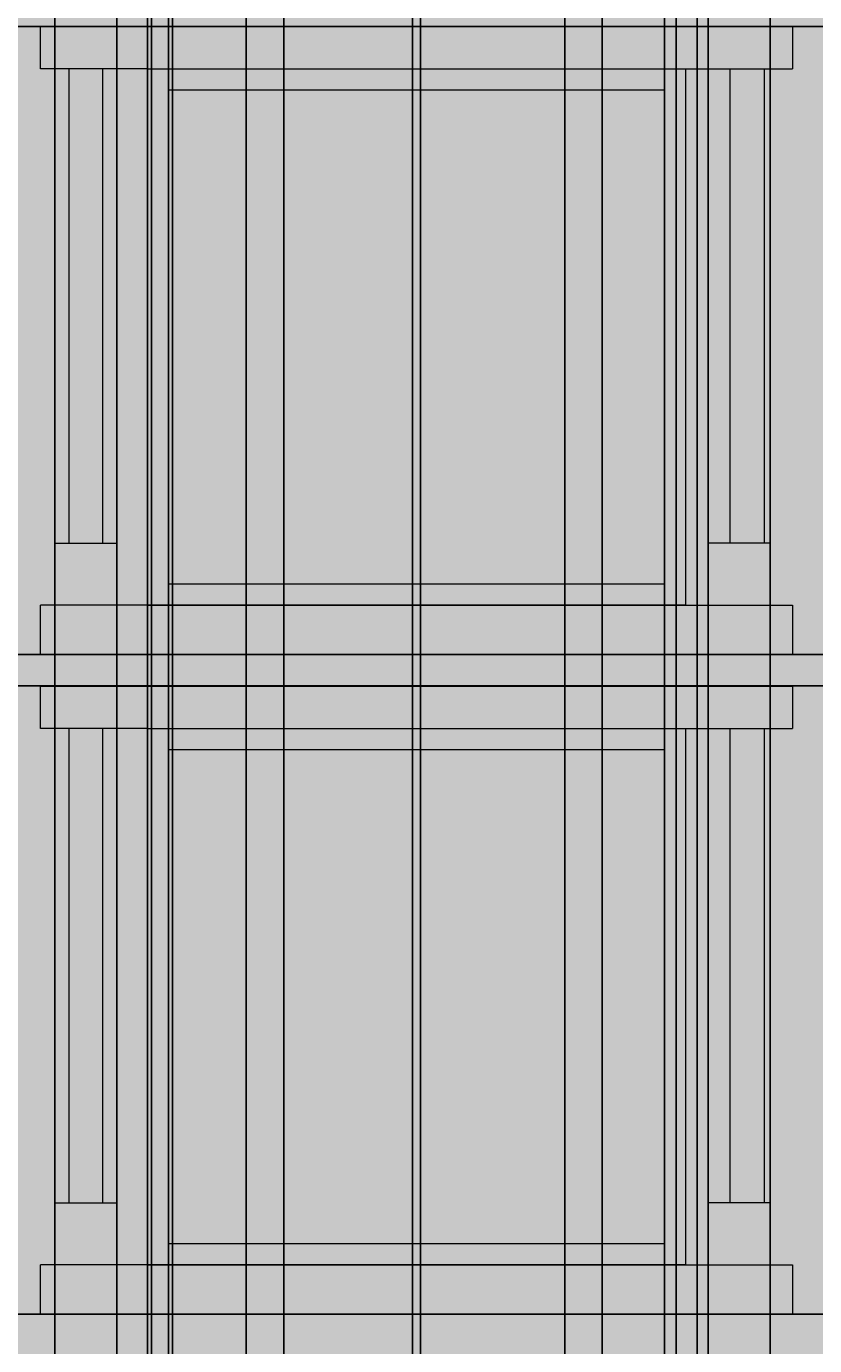
# Model space of a CAD drawing. Units: inches. Extents: x 3024 to 4744, y 1110 to 2100.
# Tile 12 of 29: x 3146 to 3297, y 1402 to 1654. Entities that reach past the tile are written whole.
import ezdxf

# ---------------------------------------------------------------- set-up
doc = ezdxf.new("R2010")
doc.units = ezdxf.units.IN
for name, color, linetype, lineweight in [('A-ANNO-DIMS', 2, 'Continuous', 18), ('A-ELEV', 7, 'Continuous', 25), ('A-ELEV-PATT', 252, 'Continuous', 13), ('A-GLAZ', 4, 'Continuous', 18)]:
    doc.layers.add(name, color=color, linetype=linetype, lineweight=lineweight)
doc.styles.get("Standard").update_dxf_attribs({"font": 'arial.ttf'})
doc.dimstyles.get("Standard").update_dxf_attribs({"dimtxt": 0.18, "dimasz": 0.18, "dimexe": 0.18, "dimexo": 0.0625, "dimgap": 0.09, "dimtad": 0, "dimtih": 1, "dimtoh": 1, "dimdec": 1, "dimzin": 0, "dimdsep": 46, "dimlunit": 3, "dimtxsty": 'Standard', "dimcen": 0.09, "dimadec": 0, "dimazin": 0, "dimtfac": 1, "dimtdec": 1, "dimtofl": 0, "dimtmove": 0, "dimatfit": 3, "dimfxl": 1, "dimtolj": 1, "dimtzin": 0, "dimarcsym": 0})

# ---------------------------------------------------------------- blocks, each defined once
blk = doc.blocks.new('WIN-BALCONY-A')
for p, q in [((3169.4, 1897.49), (3148.97, 1897.49)), ((3169.4, 1897.49), (3148.97, 1897.49)), ((3169.4, 1897.49), (3292.61, 1897.49)), ((3169.4, 1897.49), (3292.61, 1897.49)), ((3169.4, 1795.04), (3148.97, 1795.04)), ((3169.4, 1795.04), (3148.97, 1795.04)), ((3169.4, 1795.04), (3292.61, 1795.04)), ((3169.4, 1795.04), (3292.61, 1795.04))]:
    blk.add_line(p, q)
for points in [[(3148.97, 1897.49), (3148.97, 1905.61), (3292.61, 1905.61), (3292.61, 1897.49)], [(3148.97, 1897.49), (3148.97, 1905.61), (3292.61, 1905.61), (3292.61, 1897.49)], [(3292.61, 1795.04), (3292.61, 1785.61), (3148.97, 1785.61), (3148.97, 1795.04)], [(3292.61, 1795.04), (3292.61, 1785.61), (3148.97, 1785.61), (3148.97, 1795.04)]]:
    blk.add_lwpolyline(points)
for points in [[(3154.33, 1806.87), (3160.86, 1806.87), (3160.86, 1897.49), (3154.33, 1897.49)], [(3154.33, 1806.87), (3160.86, 1806.87), (3160.86, 1897.49), (3154.33, 1897.49)], [(3272.18, 1795.04), (3169.4, 1795.04), (3169.4, 1897.49), (3272.18, 1897.49)], [(3272.18, 1795.04), (3169.4, 1795.04), (3169.4, 1897.49), (3272.18, 1897.49)], [(3287.25, 1806.87), (3280.72, 1806.87), (3280.72, 1897.49), (3287.25, 1897.49)], [(3287.25, 1806.87), (3280.72, 1806.87), (3280.72, 1897.49), (3287.25, 1897.49)], [(3268.18, 1799.04), (3173.4, 1799.04), (3173.4, 1893.49), (3268.18, 1893.49)], [(3268.18, 1799.04), (3173.4, 1799.04), (3173.4, 1893.49), (3268.18, 1893.49)], [(3220.05, 1893.49), (3221.52, 1893.49), (3221.52, 1799.04), (3220.05, 1799.04)], [(3220.05, 1893.49), (3221.52, 1893.49), (3221.52, 1799.04), (3220.05, 1799.04)], [(3163.53, 1795.04), (3151.66, 1795.04), (3151.66, 1806.87), (3163.53, 1806.87)], [(3163.53, 1795.04), (3151.66, 1795.04), (3151.66, 1806.87), (3163.53, 1806.87)], [(3276.51, 1795.04), (3288.38, 1795.04), (3288.38, 1806.87), (3276.51, 1806.87)], [(3276.51, 1795.04), (3288.38, 1795.04), (3288.38, 1806.87), (3276.51, 1806.87)]]:
    blk.add_lwpolyline(points, close=True)
blk = doc.blocks.new('*D64')
at = {"layer": 'A-ANNO-DIMS', "color": 0, "lineweight": -2, "transparency": 16777216}
for p, q in [((3069.79, 1241.5), (3069.79, 2100.44)), ((3069.97, 2100.26), (3405.08, 2100.26)), ((3740.97, 2100.26), (3405.87, 2100.26)), ((3741.15, 1241.5), (3741.15, 2100.44))]:
    blk.add_line(p, q, dxfattribs=at)
at = {"layer": 'A-ANNO-DIMS', "color": 0, "transparency": 16777216}
for points in [[(3069.97, 2100.29), (3069.97, 2100.23), (3069.79, 2100.26)], [(3740.97, 2100.29), (3740.97, 2100.23), (3741.15, 2100.26)]]:
    blk.add_solid(points, dxfattribs=at)
at = {"layer": 'Defpoints', "color": 0, "transparency": 16777216}
for p in [(3741.15, 2100.26), (3069.79, 1241.43), (3741.15, 1241.43)]:
    blk.add_point(p, dxfattribs=at)
at = {"layer": 'A-ANNO-DIMS', "color": 0, "transparency": 16777216, "insert": (3405.47, 2100.26), "char_height": 0.18, "attachment_point": 5}
blk.add_mtext('\\A1;671.4', dxfattribs=at)
blk = doc.blocks.new('*D89')
at = {"layer": 'A-ANNO-DIMS', "color": 0, "lineweight": -2, "transparency": 16777216}
for p, q in [((3151.66, 1794.98), (3151.66, 1109.93)), ((3163.53, 1794.98), (3163.53, 1109.93)), ((3151.84, 1110.11), (3157.14, 1110.11)), ((3163.35, 1110.11), (3158.05, 1110.11))]:
    blk.add_line(p, q, dxfattribs=at)
at = {"layer": 'A-ANNO-DIMS', "color": 0, "transparency": 16777216}
for points in [[(3151.84, 1110.14), (3151.84, 1110.08), (3151.66, 1110.11)], [(3163.35, 1110.14), (3163.35, 1110.08), (3163.53, 1110.11)]]:
    blk.add_solid(points, dxfattribs=at)
at = {"layer": 'Defpoints', "color": 0, "transparency": 16777216}
for p in [(3151.66, 1795.04), (3163.53, 1795.04), (3163.53, 1110.11)]:
    blk.add_point(p, dxfattribs=at)
at = {"layer": 'A-ANNO-DIMS', "color": 0, "transparency": 16777216, "insert": (3157.59, 1110.11), "char_height": 0.18, "attachment_point": 5}
blk.add_mtext('\\A1;11.866', dxfattribs=at)
blk = doc.blocks.new('*D90')
at = {"layer": 'A-ANNO-DIMS', "color": 0, "lineweight": -2, "transparency": 16777216}
for p, q in [((3173.4, 1798.98), (3173.4, 1109.93)), ((3169.4, 1794.98), (3169.4, 1109.93)), ((3169.58, 1110.11), (3171.07, 1110.11)), ((3173.22, 1110.11), (3171.72, 1110.11))]:
    blk.add_line(p, q, dxfattribs=at)
at = {"layer": 'A-ANNO-DIMS', "color": 0, "transparency": 16777216}
for points in [[(3169.58, 1110.14), (3169.58, 1110.08), (3169.4, 1110.11)], [(3173.22, 1110.14), (3173.22, 1110.08), (3173.4, 1110.11)]]:
    blk.add_solid(points, dxfattribs=at)
at = {"layer": 'Defpoints', "color": 0, "transparency": 16777216}
for p in [(3173.4, 1799.04), (3169.4, 1795.04), (3173.4, 1110.11)]:
    blk.add_point(p, dxfattribs=at)
at = {"layer": 'A-ANNO-DIMS', "color": 0, "transparency": 16777216, "insert": (3171.4, 1110.11), "char_height": 0.18, "attachment_point": 5}
blk.add_mtext('\\A1;4.00', dxfattribs=at)
blk = doc.blocks.new('*D91')
at = {"layer": 'A-ANNO-DIMS', "color": 0, "lineweight": -2, "transparency": 16777216}
for p, q in [((3173.4, 1798.98), (3173.4, 1109.93)), ((3220.05, 1798.98), (3220.05, 1109.93)), ((3173.58, 1110.11), (3196.33, 1110.11)), ((3219.87, 1110.11), (3197.12, 1110.11))]:
    blk.add_line(p, q, dxfattribs=at)
at = {"layer": 'A-ANNO-DIMS', "color": 0, "transparency": 16777216}
for points in [[(3173.58, 1110.14), (3173.58, 1110.08), (3173.4, 1110.11)], [(3219.87, 1110.14), (3219.87, 1110.08), (3220.05, 1110.11)]]:
    blk.add_solid(points, dxfattribs=at)
at = {"layer": 'Defpoints', "color": 0, "transparency": 16777216}
for p in [(3173.4, 1799.04), (3220.05, 1799.04), (3220.05, 1110.11)]:
    blk.add_point(p, dxfattribs=at)
at = {"layer": 'A-ANNO-DIMS', "color": 0, "transparency": 16777216, "insert": (3196.72, 1110.11), "char_height": 0.18, "attachment_point": 5}
blk.add_mtext('\\A1;46.65', dxfattribs=at)
blk = doc.blocks.new('*D92')
at = {"layer": 'A-ANNO-DIMS', "color": 0, "lineweight": -2, "transparency": 16777216}
for p, q in [((3220.05, 1798.98), (3220.05, 1109.93)), ((3221.52, 1798.98), (3221.52, 1109.93)), ((3220.23, 1110.11), (3220.47, 1110.11)), ((3221.34, 1110.11), (3221.1, 1110.11))]:
    blk.add_line(p, q, dxfattribs=at)
at = {"layer": 'A-ANNO-DIMS', "color": 0, "transparency": 16777216}
for points in [[(3220.23, 1110.14), (3220.23, 1110.08), (3220.05, 1110.11)], [(3221.34, 1110.14), (3221.34, 1110.08), (3221.52, 1110.11)]]:
    blk.add_solid(points, dxfattribs=at)
at = {"layer": 'Defpoints', "color": 0, "transparency": 16777216}
for p in [(3220.05, 1799.04), (3221.52, 1799.04), (3221.52, 1110.11)]:
    blk.add_point(p, dxfattribs=at)
at = {"layer": 'A-ANNO-DIMS', "color": 0, "transparency": 16777216, "insert": (3220.79, 1110.11), "char_height": 0.18, "attachment_point": 5}
blk.add_mtext('\\A1;1.47', dxfattribs=at)
blk = doc.blocks.new('*D93')
at = {"layer": 'A-ANNO-DIMS', "color": 0, "lineweight": -2, "transparency": 16777216}
for p, q in [((3221.52, 1798.98), (3221.52, 1109.93)), ((3268.18, 1798.98), (3268.18, 1109.93)), ((3221.7, 1110.11), (3244.45, 1110.11)), ((3268, 1110.11), (3245.25, 1110.11))]:
    blk.add_line(p, q, dxfattribs=at)
at = {"layer": 'A-ANNO-DIMS', "color": 0, "transparency": 16777216}
for points in [[(3221.7, 1110.14), (3221.7, 1110.08), (3221.52, 1110.11)], [(3268, 1110.14), (3268, 1110.08), (3268.18, 1110.11)]]:
    blk.add_solid(points, dxfattribs=at)
at = {"layer": 'Defpoints', "color": 0, "transparency": 16777216}
for p in [(3221.52, 1799.04), (3268.18, 1799.04), (3268.18, 1110.11)]:
    blk.add_point(p, dxfattribs=at)
at = {"layer": 'A-ANNO-DIMS', "color": 0, "transparency": 16777216, "insert": (3244.85, 1110.11), "char_height": 0.18, "attachment_point": 5}
blk.add_mtext('\\A1;46.65', dxfattribs=at)
blk = doc.blocks.new('*D94')
at = {"layer": 'A-ANNO-DIMS', "color": 0, "lineweight": -2, "transparency": 16777216}
for p, q in [((3276.51, 1794.98), (3276.51, 1109.93)), ((3288.38, 1794.98), (3288.38, 1109.93)), ((3276.69, 1110.11), (3281.99, 1110.11)), ((3288.2, 1110.11), (3282.9, 1110.11))]:
    blk.add_line(p, q, dxfattribs=at)
at = {"layer": 'A-ANNO-DIMS', "color": 0, "transparency": 16777216}
for points in [[(3276.69, 1110.14), (3276.69, 1110.08), (3276.51, 1110.11)], [(3288.2, 1110.14), (3288.2, 1110.08), (3288.38, 1110.11)]]:
    blk.add_solid(points, dxfattribs=at)
at = {"layer": 'Defpoints', "color": 0, "transparency": 16777216}
for p in [(3276.51, 1795.04), (3288.38, 1795.04), (3288.38, 1110.11)]:
    blk.add_point(p, dxfattribs=at)
at = {"layer": 'A-ANNO-DIMS', "color": 0, "transparency": 16777216, "insert": (3282.44, 1110.11), "char_height": 0.18, "attachment_point": 5}
blk.add_mtext('\\A1;11.866', dxfattribs=at)
blk = doc.blocks.new('*D106')
at = {"layer": 'A-ANNO-DIMS', "color": 0, "lineweight": -2, "transparency": 16777216}
for p, q in [((3170.16, 1275.67), (3170.16, 2100.44)), ((3170.34, 2100.26), (3171.83, 2100.26)), ((3173.98, 2100.26), (3172.49, 2100.26)), ((3174.16, 1271.67), (3174.16, 2100.44))]:
    blk.add_line(p, q, dxfattribs=at)
at = {"layer": 'A-ANNO-DIMS', "color": 0, "transparency": 16777216}
for points in [[(3170.34, 2100.29), (3170.34, 2100.23), (3170.16, 2100.26)], [(3173.98, 2100.29), (3173.98, 2100.23), (3174.16, 2100.26)]]:
    blk.add_solid(points, dxfattribs=at)
at = {"layer": 'Defpoints', "color": 0, "transparency": 16777216}
for p in [(3174.16, 2100.26), (3170.16, 1275.61), (3174.16, 1271.61)]:
    blk.add_point(p, dxfattribs=at)
at = {"layer": 'A-ANNO-DIMS', "color": 0, "transparency": 16777216, "insert": (3172.16, 2100.26), "char_height": 0.18, "attachment_point": 5}
blk.add_mtext('\\A1;4.00', dxfattribs=at)
blk = doc.blocks.new('*D107')
at = {"layer": 'A-ANNO-DIMS', "color": 0, "lineweight": -2, "transparency": 16777216}
for p, q in [((3174.16, 1271.67), (3174.16, 2100.44)), ((3174.34, 2100.26), (3221.88, 2100.26)), ((3270.21, 2100.26), (3222.67, 2100.26)), ((3270.39, 1271.67), (3270.39, 2100.44))]:
    blk.add_line(p, q, dxfattribs=at)
at = {"layer": 'A-ANNO-DIMS', "color": 0, "transparency": 16777216}
for points in [[(3174.34, 2100.29), (3174.34, 2100.23), (3174.16, 2100.26)], [(3270.21, 2100.29), (3270.21, 2100.23), (3270.39, 2100.26)]]:
    blk.add_solid(points, dxfattribs=at)
at = {"layer": 'Defpoints', "color": 0, "transparency": 16777216}
for p in [(3270.39, 2100.26), (3174.16, 1271.61), (3270.39, 1271.61)]:
    blk.add_point(p, dxfattribs=at)
at = {"layer": 'A-ANNO-DIMS', "color": 0, "transparency": 16777216, "insert": (3222.27, 2100.26), "char_height": 0.18, "attachment_point": 5}
blk.add_mtext('\\A1;96.23', dxfattribs=at)
blk = doc.blocks.new('*D108')
at = {"layer": 'A-ANNO-DIMS', "color": 0, "lineweight": -2, "transparency": 16777216}
for p, q in [((3270.39, 1271.67), (3270.39, 2100.44)), ((3270.57, 2100.26), (3272.06, 2100.26)), ((3274.21, 2100.26), (3272.71, 2100.26)), ((3274.39, 1275.67), (3274.39, 2100.44))]:
    blk.add_line(p, q, dxfattribs=at)
at = {"layer": 'A-ANNO-DIMS', "color": 0, "transparency": 16777216}
for points in [[(3270.57, 2100.29), (3270.57, 2100.23), (3270.39, 2100.26)], [(3274.21, 2100.29), (3274.21, 2100.23), (3274.39, 2100.26)]]:
    blk.add_solid(points, dxfattribs=at)
at = {"layer": 'Defpoints', "color": 0, "transparency": 16777216}
for p in [(3274.39, 2100.26), (3274.39, 1275.61), (3270.39, 1271.61)]:
    blk.add_point(p, dxfattribs=at)
at = {"layer": 'A-ANNO-DIMS', "color": 0, "transparency": 16777216, "insert": (3272.39, 2100.26), "char_height": 0.18, "attachment_point": 5}
blk.add_mtext('\\A1;4.00', dxfattribs=at)
blk = doc.blocks.new('*D124')
at = {"layer": 'A-ANNO-DIMS', "color": 0, "lineweight": -2, "transparency": 16777216}
for p, q in [((3174.16, 1271.67), (3174.16, 2100.44)), ((3174.34, 2100.26), (3180.75, 2100.26)), ((3188.08, 2100.26), (3181.67, 2100.26)), ((3188.26, 1256.29), (3188.26, 2100.44))]:
    blk.add_line(p, q, dxfattribs=at)
at = {"layer": 'A-ANNO-DIMS', "color": 0, "transparency": 16777216}
for points in [[(3174.34, 2100.29), (3174.34, 2100.23), (3174.16, 2100.26)], [(3188.08, 2100.29), (3188.08, 2100.23), (3188.26, 2100.26)]]:
    blk.add_solid(points, dxfattribs=at)
at = {"layer": 'Defpoints', "color": 0, "transparency": 16777216}
for p in [(3188.26, 2100.26), (3174.16, 1271.61), (3188.26, 1256.23)]:
    blk.add_point(p, dxfattribs=at)
at = {"layer": 'A-ANNO-DIMS', "color": 0, "transparency": 16777216, "insert": (3181.21, 2100.26), "char_height": 0.18, "attachment_point": 5}
blk.add_mtext('\\A1;14.098', dxfattribs=at)
blk = doc.blocks.new('*D125')
at = {"layer": 'A-ANNO-DIMS', "color": 0, "lineweight": -2, "transparency": 16777216}
for p, q in [((3188.26, 1256.29), (3188.26, 2100.44)), ((3188.44, 2100.26), (3191.44, 2100.26)), ((3195.23, 2100.26), (3192.22, 2100.26)), ((3195.41, 1256.29), (3195.41, 2100.44))]:
    blk.add_line(p, q, dxfattribs=at)
at = {"layer": 'A-ANNO-DIMS', "color": 0, "transparency": 16777216}
for points in [[(3188.44, 2100.29), (3188.44, 2100.23), (3188.26, 2100.26)], [(3195.23, 2100.29), (3195.23, 2100.23), (3195.41, 2100.26)]]:
    blk.add_solid(points, dxfattribs=at)
at = {"layer": 'Defpoints', "color": 0, "transparency": 16777216}
for p in [(3195.41, 2100.26), (3188.26, 1256.23), (3195.41, 1256.23)]:
    blk.add_point(p, dxfattribs=at)
at = {"layer": 'A-ANNO-DIMS', "color": 0, "transparency": 16777216, "insert": (3191.83, 2100.26), "char_height": 0.18, "attachment_point": 5}
blk.add_mtext('\\A1;7.147', dxfattribs=at)
blk = doc.blocks.new('*D126')
at = {"layer": 'A-ANNO-DIMS', "color": 0, "lineweight": -2, "transparency": 16777216}
for p, q in [((3249.14, 1256.29), (3249.14, 2100.44)), ((3249.32, 2100.26), (3252.32, 2100.26)), ((3256.11, 2100.26), (3253.11, 2100.26)), ((3256.29, 1256.29), (3256.29, 2100.44))]:
    blk.add_line(p, q, dxfattribs=at)
at = {"layer": 'A-ANNO-DIMS', "color": 0, "transparency": 16777216}
for points in [[(3249.32, 2100.29), (3249.32, 2100.23), (3249.14, 2100.26)], [(3256.11, 2100.29), (3256.11, 2100.23), (3256.29, 2100.26)]]:
    blk.add_solid(points, dxfattribs=at)
at = {"layer": 'Defpoints', "color": 0, "transparency": 16777216}
for p in [(3256.29, 2100.26), (3249.14, 1256.23), (3256.29, 1256.23)]:
    blk.add_point(p, dxfattribs=at)
at = {"layer": 'A-ANNO-DIMS', "color": 0, "transparency": 16777216, "insert": (3252.72, 2100.26), "char_height": 0.18, "attachment_point": 5}
blk.add_mtext('\\A1;7.147', dxfattribs=at)

msp = doc.modelspace()

# ---------------------------------------------------------------- hatches: boundary and pattern name
at = {"layer": 'A-ELEV-PATT'}
h = msp.add_hatch(color=256, dxfattribs=at)
h.dxf.hatch_style = 1
h.paths.add_polyline_path([(3491.8271, 2054.7584), (3320.5658, 2054.7584), (3320.5658, 2043.5286), (3491.8271, 2043.5286)])
h.paths.add_polyline_path([(3292.6051, 1905.6112), (3148.9694, 1905.6112), (3148.9694, 1897.4879), (3169.3964, 1897.4879), (3292.6051, 1897.4879)])
h.paths.add_polyline_path([(3292.6051, 1795.0431), (3169.3964, 1795.0431), (3148.9694, 1795.0431), (3148.9694, 1785.6112), (3292.6051, 1785.6112)])
h.paths.add_polyline_path([(3292.6051, 1779.6112), (3148.9694, 1779.6112), (3148.9694, 1771.4879), (3169.3964, 1771.4879), (3292.6051, 1771.4879)])
h.paths.add_polyline_path([(3292.6051, 1669.0431), (3169.3964, 1669.0431), (3148.9694, 1669.0431), (3148.9694, 1659.6112), (3292.6051, 1659.6112)])
h.paths.add_polyline_path([(3292.6051, 1653.6112), (3148.9694, 1653.6112), (3148.9694, 1645.4879), (3169.3964, 1645.4879), (3292.6051, 1645.4879)])
h.paths.add_polyline_path([(3292.6051, 1543.0431), (3169.3964, 1543.0431), (3148.9694, 1543.0431), (3148.9694, 1533.6112), (3292.6051, 1533.6112)])
h.paths.add_polyline_path([(3292.6051, 1527.6112), (3148.9694, 1527.6112), (3148.9694, 1519.4879), (3169.3964, 1519.4879), (3292.6051, 1519.4879)])
h.paths.add_polyline_path([(3292.6051, 1401.6112), (3148.9694, 1401.6112), (3148.9694, 1393.4879), (3169.3964, 1393.4879), (3292.6051, 1393.4879)])
h.paths.add_polyline_path([(3292.6051, 1417.0431), (3169.3964, 1417.0431), (3148.9694, 1417.0431), (3148.9694, 1407.6112), (3292.6051, 1407.6112)])
h.paths.add_polyline_path([(3292.6051, 1291.0431), (3169.3964, 1291.0431), (3148.9694, 1291.0431), (3148.9694, 1281.6112), (3292.6051, 1281.6112)])
h.paths.add_polyline_path([(3654.037, 1165.0431), (3530.8283, 1165.0431), (3510.4013, 1165.0431), (3510.4013, 1155.6112), (3654.037, 1155.6112)])
h.paths.add_polyline_path([(3654.037, 1275.6112), (3510.4013, 1275.6112), (3510.4013, 1267.4879), (3530.8283, 1267.4879), (3654.037, 1267.4879)])
h.paths.add_polyline_path([(3654.037, 1291.0431), (3530.8283, 1291.0431), (3510.4013, 1291.0431), (3510.4013, 1281.6112), (3654.037, 1281.6112)])
h.paths.add_polyline_path([(3654.037, 1417.0431), (3530.8283, 1417.0431), (3510.4013, 1417.0431), (3510.4013, 1407.6112), (3654.037, 1407.6112)])
h.paths.add_polyline_path([(3654.037, 1401.6112), (3510.4013, 1401.6112), (3510.4013, 1393.4879), (3530.8283, 1393.4879), (3654.037, 1393.4879)])
h.paths.add_polyline_path([(3654.037, 1543.0431), (3530.8283, 1543.0431), (3510.4013, 1543.0431), (3510.4013, 1533.6112), (3654.037, 1533.6112)])
h.paths.add_polyline_path([(3654.037, 1527.6112), (3510.4013, 1527.6112), (3510.4013, 1519.4879), (3530.8283, 1519.4879), (3654.037, 1519.4879)])
h.paths.add_polyline_path([(3654.037, 1653.6112), (3510.4013, 1653.6112), (3510.4013, 1645.4879), (3530.8283, 1645.4879), (3654.037, 1645.4879)])
h.paths.add_polyline_path([(3654.037, 1669.0431), (3530.8283, 1669.0431), (3510.4013, 1669.0431), (3510.4013, 1659.6112), (3654.037, 1659.6112)])
h.paths.add_polyline_path([(3654.037, 1779.6112), (3510.4013, 1779.6112), (3510.4013, 1771.4879), (3530.8283, 1771.4879), (3654.037, 1771.4879)])
h.paths.add_polyline_path([(3654.037, 1795.0431), (3530.8283, 1795.0431), (3510.4013, 1795.0431), (3510.4013, 1785.6112), (3654.037, 1785.6112)])
h.paths.add_polyline_path([(3654.037, 1905.6112), (3510.4013, 1905.6112), (3510.4013, 1897.4879), (3530.8283, 1897.4879), (3654.037, 1897.4879)])
h = msp.add_hatch(color=256, dxfattribs=at)
h.dxf.hatch_style = 1
h.paths.add_polyline_path([(3329.7033, 1407.6112), (3105.4722, 1407.6112), (3105.4722, 1401.6112), (3329.7033, 1401.6112)])
h.paths.add_polyline_path([(3329.7033, 1281.6112), (3105.4722, 1281.6112), (3105.4722, 1275.6112), (3112.3838, 1275.6112), (3329.7033, 1275.6112)])
h.paths.add_polyline_path([(3329.7033, 1533.6112), (3105.4722, 1533.6112), (3105.4722, 1527.6112), (3329.7033, 1527.6112)])
h.paths.add_polyline_path([(3329.7033, 1659.6112), (3105.4722, 1659.6112), (3105.4722, 1653.6112), (3329.7033, 1653.6112)])
h.paths.add_polyline_path([(3329.7033, 1785.6112), (3105.4722, 1785.6112), (3105.4722, 1779.6112), (3329.7033, 1779.6112)])
h.paths.add_polyline_path([(3329.7033, 1911.6112), (3105.4722, 1911.6112), (3095.7158, 1911.6112), (3095.7158, 1905.6112), (3329.7033, 1905.6112)])
h.paths.add_polyline_path([(3715.2286, 1911.6112), (3705.4722, 1911.6112), (3705.4722, 1905.6112), (3715.2286, 1905.6112)])
h.paths.add_polyline_path([(3688.5588, 1911.6112), (3481.2411, 1911.6112), (3481.2411, 1905.6112), (3688.5588, 1905.6112)])
h = msp.add_hatch(color=256, dxfattribs=at)
h.dxf.hatch_style = 1
h.paths.add_polyline_path([(3154.3287, 1897.4879), (3148.9694, 1897.4879), (3148.9694, 1905.6112), (3105.4722, 1905.6112), (3105.4722, 1785.6112), (3148.9694, 1785.6112), (3148.9694, 1795.0431), (3151.6604, 1795.0431), (3151.6604, 1806.8674), (3154.3287, 1806.8674)])
h.paths.add_polyline_path([(3329.7033, 1905.6112), (3292.6051, 1905.6112), (3292.6051, 1897.4879), (3287.2458, 1897.4879), (3287.2458, 1806.8674), (3288.3759, 1806.8674), (3288.3759, 1795.0431), (3292.6051, 1795.0431), (3292.6051, 1785.6112), (3329.7033, 1785.6112)])
h.paths.add_polyline_path([(3154.3287, 1771.4879), (3148.9694, 1771.4879), (3148.9694, 1779.6112), (3105.4722, 1779.6112), (3105.4722, 1659.6112), (3148.9694, 1659.6112), (3148.9694, 1669.0431), (3151.6604, 1669.0431), (3151.6604, 1680.8674), (3154.3287, 1680.8674)])
h.paths.add_polyline_path([(3329.7033, 1779.6112), (3292.6051, 1779.6112), (3292.6051, 1771.4879), (3287.2458, 1771.4879), (3287.2458, 1680.8674), (3288.3759, 1680.8674), (3288.3759, 1669.0431), (3292.6051, 1669.0431), (3292.6051, 1659.6112), (3329.7033, 1659.6112)])
h.paths.add_polyline_path([(3154.3287, 1645.4879), (3148.9694, 1645.4879), (3148.9694, 1653.6112), (3105.4722, 1653.6112), (3105.4722, 1533.6112), (3148.9694, 1533.6112), (3148.9694, 1543.0431), (3151.6604, 1543.0431), (3151.6604, 1554.8674), (3154.3287, 1554.8674)])
h.paths.add_polyline_path([(3329.7033, 1653.6112), (3292.6051, 1653.6112), (3292.6051, 1645.4879), (3287.2458, 1645.4879), (3287.2458, 1554.8674), (3288.3759, 1554.8674), (3288.3759, 1543.0431), (3292.6051, 1543.0431), (3292.6051, 1533.6112), (3329.7033, 1533.6112)])
h.paths.add_polyline_path([(3329.7033, 1527.6112), (3292.6051, 1527.6112), (3292.6051, 1519.4879), (3287.2458, 1519.4879), (3287.2458, 1428.8674), (3288.3759, 1428.8674), (3288.3759, 1417.0431), (3292.6051, 1417.0431), (3292.6051, 1407.6112), (3329.7033, 1407.6112)])
h.paths.add_polyline_path([(3329.7033, 1401.6112), (3292.6051, 1401.6112), (3292.6051, 1393.4879), (3287.2458, 1393.4879), (3287.2458, 1302.8674), (3288.3759, 1302.8674), (3288.3759, 1291.0431), (3292.6051, 1291.0431), (3292.6051, 1281.6112), (3329.7033, 1281.6112)])
h.paths.add_polyline_path([(3154.3287, 1393.4879), (3148.9694, 1393.4879), (3148.9694, 1401.6112), (3105.4722, 1401.6112), (3105.4722, 1281.6112), (3148.9694, 1281.6112), (3148.9694, 1291.0431), (3151.6604, 1291.0431), (3151.6604, 1302.8674), (3154.3287, 1302.8674)])
h.paths.add_polyline_path([(3154.3287, 1519.4879), (3148.9694, 1519.4879), (3148.9694, 1527.6112), (3105.4722, 1527.6112), (3105.4722, 1407.6112), (3148.9694, 1407.6112), (3148.9694, 1417.0431), (3151.6604, 1417.0431), (3151.6604, 1428.8674), (3154.3287, 1428.8674)])
h.paths.add_polyline_path([(3515.7606, 1897.4879), (3510.4013, 1897.4879), (3510.4013, 1905.6112), (3481.2411, 1905.6112), (3481.2411, 1785.6112), (3510.4013, 1785.6112), (3510.4013, 1795.0431), (3513.0923, 1795.0431), (3513.0923, 1806.8674), (3515.7606, 1806.8674)])
h.paths.add_polyline_path([(3688.5588, 1905.6112), (3654.037, 1905.6112), (3654.037, 1897.4879), (3648.6777, 1897.4879), (3648.6777, 1806.8674), (3649.8078, 1806.8674), (3649.8078, 1795.0431), (3654.037, 1795.0431), (3654.037, 1785.6112), (3688.5588, 1785.6112)])
h.paths.add_polyline_path([(3515.7606, 1771.4879), (3510.4013, 1771.4879), (3510.4013, 1779.6112), (3481.2411, 1779.6112), (3481.2411, 1659.6112), (3510.4013, 1659.6112), (3510.4013, 1669.0431), (3513.0923, 1669.0431), (3513.0923, 1680.8674), (3515.7606, 1680.8674)])
h.paths.add_polyline_path([(3688.5588, 1779.6112), (3654.037, 1779.6112), (3654.037, 1771.4879), (3648.6777, 1771.4879), (3648.6777, 1680.8674), (3649.8078, 1680.8674), (3649.8078, 1669.0431), (3654.037, 1669.0431), (3654.037, 1659.6112), (3688.5588, 1659.6112)])
h.paths.add_polyline_path([(3515.7606, 1645.4879), (3510.4013, 1645.4879), (3510.4013, 1653.6112), (3481.2411, 1653.6112), (3481.2411, 1533.6112), (3510.4013, 1533.6112), (3510.4013, 1543.0431), (3513.0923, 1543.0431), (3513.0923, 1554.8674), (3515.7606, 1554.8674)])
h.paths.add_polyline_path([(3688.5588, 1653.6112), (3654.037, 1653.6112), (3654.037, 1645.4879), (3648.6777, 1645.4879), (3648.6777, 1554.8674), (3649.8078, 1554.8674), (3649.8078, 1543.0431), (3654.037, 1543.0431), (3654.037, 1533.6112), (3688.5588, 1533.6112)])
h.paths.add_polyline_path([(3515.7606, 1519.4879), (3510.4013, 1519.4879), (3510.4013, 1527.6112), (3481.2411, 1527.6112), (3481.2411, 1407.6112), (3510.4013, 1407.6112), (3510.4013, 1417.0431), (3513.0923, 1417.0431), (3513.0923, 1428.8674), (3515.7606, 1428.8674)])
h.paths.add_polyline_path([(3688.5588, 1527.6112), (3654.037, 1527.6112), (3654.037, 1519.4879), (3648.6777, 1519.4879), (3648.6777, 1428.8674), (3649.8078, 1428.8674), (3649.8078, 1417.0431), (3654.037, 1417.0431), (3654.037, 1407.6112), (3688.5588, 1407.6112)])
h.paths.add_polyline_path([(3515.7606, 1393.4879), (3510.4013, 1393.4879), (3510.4013, 1401.6112), (3481.2411, 1401.6112), (3481.2411, 1281.6112), (3510.4013, 1281.6112), (3510.4013, 1291.0431), (3513.0923, 1291.0431), (3513.0923, 1302.8674), (3515.7606, 1302.8674)])
h.paths.add_polyline_path([(3688.5588, 1401.6112), (3654.037, 1401.6112), (3654.037, 1393.4879), (3648.6777, 1393.4879), (3648.6777, 1302.8674), (3649.8078, 1302.8674), (3649.8078, 1291.0431), (3654.037, 1291.0431), (3654.037, 1281.6112), (3688.5588, 1281.6112)])
h.paths.add_polyline_path([(3515.7606, 1267.4879), (3510.4013, 1267.4879), (3510.4013, 1275.6112), (3481.2411, 1275.6112), (3481.2411, 1155.6112), (3510.4013, 1155.6112), (3510.4013, 1165.0431), (3513.0923, 1165.0431), (3513.0923, 1176.8674), (3515.7606, 1176.8674)])
h.paths.add_polyline_path([(3688.5588, 1275.6112), (3654.037, 1275.6112), (3654.037, 1267.4879), (3648.6777, 1267.4879), (3648.6777, 1176.8674), (3649.8078, 1176.8674), (3649.8078, 1165.0431), (3654.037, 1165.0431), (3654.037, 1155.6112), (3688.5588, 1155.6112)])
h.paths.add_polyline_path([(3112.3838, 1275.6112), (3105.4722, 1275.6112), (3105.4722, 1171.0239), (3112.3838, 1171.0239)])
h = msp.add_hatch(color=256, dxfattribs=at)
h.dxf.hatch_style = 1
h.paths.add_polyline_path([(3160.8586, 1897.4879), (3154.3287, 1897.4879), (3154.3287, 1806.8674), (3160.8586, 1806.8674)])
h.paths.add_polyline_path([(3287.2458, 1897.4879), (3280.716, 1897.4879), (3280.716, 1806.8674), (3287.2458, 1806.8674)])
h.paths.add_polyline_path([(3160.8586, 1771.4879), (3154.3287, 1771.4879), (3154.3287, 1680.8674), (3160.8586, 1680.8674)])
h.paths.add_polyline_path([(3287.2458, 1771.4879), (3280.716, 1771.4879), (3280.716, 1680.8674), (3287.2458, 1680.8674)])
h.paths.add_polyline_path([(3160.8586, 1645.4879), (3154.3287, 1645.4879), (3154.3287, 1554.8674), (3160.8586, 1554.8674)])
h.paths.add_polyline_path([(3287.2458, 1645.4879), (3280.716, 1645.4879), (3280.716, 1554.8674), (3287.2458, 1554.8674)])
h.paths.add_polyline_path([(3160.8586, 1519.4879), (3154.3287, 1519.4879), (3154.3287, 1428.8674), (3160.8586, 1428.8674)])
h.paths.add_polyline_path([(3287.2458, 1519.4879), (3280.716, 1519.4879), (3280.716, 1428.8674), (3287.2458, 1428.8674)])
h.paths.add_polyline_path([(3160.8586, 1393.4879), (3154.3287, 1393.4879), (3154.3287, 1302.8674), (3160.8586, 1302.8674)])
h.paths.add_polyline_path([(3287.2458, 1393.4879), (3280.716, 1393.4879), (3280.716, 1302.8674), (3287.2458, 1302.8674)])
h.paths.add_polyline_path([(3648.6777, 1267.4879), (3642.1479, 1267.4879), (3642.1479, 1176.8674), (3648.6777, 1176.8674)])
h.paths.add_polyline_path([(3522.2905, 1267.4879), (3515.7606, 1267.4879), (3515.7606, 1176.8674), (3522.2905, 1176.8674)])
h.paths.add_polyline_path([(3522.2905, 1393.4879), (3515.7606, 1393.4879), (3515.7606, 1302.8674), (3522.2905, 1302.8674)])
h.paths.add_polyline_path([(3648.6777, 1393.4879), (3642.1479, 1393.4879), (3642.1479, 1302.8674), (3648.6777, 1302.8674)])
h.paths.add_polyline_path([(3522.2905, 1519.4879), (3515.7606, 1519.4879), (3515.7606, 1428.8674), (3522.2905, 1428.8674)])
h.paths.add_polyline_path([(3648.6777, 1519.4879), (3642.1479, 1519.4879), (3642.1479, 1428.8674), (3648.6777, 1428.8674)])
h.paths.add_polyline_path([(3522.2905, 1645.4879), (3515.7606, 1645.4879), (3515.7606, 1554.8674), (3522.2905, 1554.8674)])
h.paths.add_polyline_path([(3522.2905, 1771.4879), (3515.7606, 1771.4879), (3515.7606, 1680.8674), (3522.2905, 1680.8674)])
h.paths.add_polyline_path([(3648.6777, 1645.4879), (3642.1479, 1645.4879), (3642.1479, 1554.8674), (3648.6777, 1554.8674)])
h.paths.add_polyline_path([(3648.6777, 1771.4879), (3642.1479, 1771.4879), (3642.1479, 1680.8674), (3648.6777, 1680.8674)])
h.paths.add_polyline_path([(3648.6777, 1897.4879), (3642.1479, 1897.4879), (3642.1479, 1806.8674), (3648.6777, 1806.8674)])
h.paths.add_polyline_path([(3522.2905, 1897.4879), (3515.7606, 1897.4879), (3515.7606, 1806.8674), (3522.2905, 1806.8674)])
h = msp.add_hatch(color=256, dxfattribs=at)
h.dxf.hatch_style = 1
h.paths.add_polyline_path([(3169.3964, 1897.4879), (3160.8586, 1897.4879), (3160.8586, 1806.8674), (3163.5269, 1806.8674), (3163.5269, 1795.0431), (3169.3964, 1795.0431)])
h.paths.add_polyline_path([(3280.716, 1897.4879), (3272.1781, 1897.4879), (3272.1781, 1795.0431), (3276.5094, 1795.0431), (3276.5094, 1806.8674), (3280.716, 1806.8674)])
h.paths.add_polyline_path([(3280.716, 1771.4879), (3272.1781, 1771.4879), (3272.1781, 1669.0431), (3276.5094, 1669.0431), (3276.5094, 1680.8674), (3280.716, 1680.8674)])
h.paths.add_polyline_path([(3169.3964, 1771.4879), (3160.8586, 1771.4879), (3160.8586, 1680.8674), (3163.5269, 1680.8674), (3163.5269, 1669.0431), (3169.3964, 1669.0431)])
h.paths.add_polyline_path([(3169.3964, 1645.4879), (3160.8586, 1645.4879), (3160.8586, 1554.8674), (3163.5269, 1554.8674), (3163.5269, 1543.0431), (3169.3964, 1543.0431)])
h.paths.add_polyline_path([(3280.716, 1645.4879), (3272.1781, 1645.4879), (3272.1781, 1543.0431), (3276.5094, 1543.0431), (3276.5094, 1554.8674), (3280.716, 1554.8674)])
h.paths.add_polyline_path([(3169.3964, 1519.4879), (3160.8586, 1519.4879), (3160.8586, 1428.8674), (3163.5269, 1428.8674), (3163.5269, 1417.0431), (3169.3964, 1417.0431)])
h.paths.add_polyline_path([(3280.716, 1519.4879), (3272.1781, 1519.4879), (3272.1781, 1417.0431), (3276.5094, 1417.0431), (3276.5094, 1428.8674), (3280.716, 1428.8674)])
h.paths.add_polyline_path([(3169.3964, 1393.4879), (3160.8586, 1393.4879), (3160.8586, 1302.8674), (3163.5269, 1302.8674), (3163.5269, 1291.0431), (3169.3964, 1291.0431)])
h.paths.add_polyline_path([(3280.716, 1393.4879), (3272.1781, 1393.4879), (3272.1781, 1291.0431), (3276.5094, 1291.0431), (3276.5094, 1302.8674), (3280.716, 1302.8674)])
h.paths.add_polyline_path([(3642.1479, 1267.4879), (3633.61, 1267.4879), (3633.61, 1165.0431), (3637.9413, 1165.0431), (3637.9413, 1176.8674), (3642.1479, 1176.8674)])
h.paths.add_polyline_path([(3530.8283, 1267.4879), (3522.2905, 1267.4879), (3522.2905, 1176.8674), (3524.9588, 1176.8674), (3524.9588, 1165.0431), (3530.8283, 1165.0431)])
h.paths.add_polyline_path([(3642.1479, 1393.4879), (3633.61, 1393.4879), (3633.61, 1291.0431), (3637.9413, 1291.0431), (3637.9413, 1302.8674), (3642.1479, 1302.8674)])
h.paths.add_polyline_path([(3530.8283, 1393.4879), (3522.2905, 1393.4879), (3522.2905, 1302.8674), (3524.9588, 1302.8674), (3524.9588, 1291.0431), (3530.8283, 1291.0431)])
h.paths.add_polyline_path([(3530.8283, 1519.4879), (3522.2905, 1519.4879), (3522.2905, 1428.8674), (3524.9588, 1428.8674), (3524.9588, 1417.0431), (3530.8283, 1417.0431)])
h.paths.add_polyline_path([(3642.1479, 1519.4879), (3633.61, 1519.4879), (3633.61, 1417.0431), (3637.9413, 1417.0431), (3637.9413, 1428.8674), (3642.1479, 1428.8674)])
h.paths.add_polyline_path([(3530.8283, 1645.4879), (3522.2905, 1645.4879), (3522.2905, 1554.8674), (3524.9588, 1554.8674), (3524.9588, 1543.0431), (3530.8283, 1543.0431)])
h.paths.add_polyline_path([(3642.1479, 1645.4879), (3633.61, 1645.4879), (3633.61, 1543.0431), (3637.9413, 1543.0431), (3637.9413, 1554.8674), (3642.1479, 1554.8674)])
h.paths.add_polyline_path([(3642.1479, 1771.4879), (3633.61, 1771.4879), (3633.61, 1669.0431), (3637.9413, 1669.0431), (3637.9413, 1680.8674), (3642.1479, 1680.8674)])
h.paths.add_polyline_path([(3530.8283, 1771.4879), (3522.2905, 1771.4879), (3522.2905, 1680.8674), (3524.9588, 1680.8674), (3524.9588, 1669.0431), (3530.8283, 1669.0431)])
h.paths.add_polyline_path([(3530.8283, 1897.4879), (3522.2905, 1897.4879), (3522.2905, 1806.8674), (3524.9588, 1806.8674), (3524.9588, 1795.0431), (3530.8283, 1795.0431)])
h.paths.add_polyline_path([(3642.1479, 1897.4879), (3633.61, 1897.4879), (3633.61, 1795.0431), (3637.9413, 1795.0431), (3637.9413, 1806.8674), (3642.1479, 1806.8674)])
h = msp.add_hatch(color=256, dxfattribs=at)
h.dxf.hatch_style = 1
h.paths.add_polyline_path([(3220.0505, 1893.4879), (3173.3964, 1893.4879), (3173.3964, 1799.0431), (3220.0505, 1799.0431)])
h.paths.add_polyline_path([(3268.1781, 1893.4879), (3221.5241, 1893.4879), (3221.5241, 1799.0431), (3268.1781, 1799.0431)])
h.paths.add_polyline_path([(3581.4824, 1893.4879), (3534.8283, 1893.4879), (3534.8283, 1799.0431), (3581.4824, 1799.0431)])
h.paths.add_polyline_path([(3629.61, 1893.4879), (3582.956, 1893.4879), (3582.956, 1799.0431), (3629.61, 1799.0431)])
h.paths.add_polyline_path([(3581.4824, 1767.4879), (3534.8283, 1767.4879), (3534.8283, 1673.0431), (3581.4824, 1673.0431)])
h.paths.add_polyline_path([(3629.61, 1767.4879), (3582.956, 1767.4879), (3582.956, 1673.0431), (3629.61, 1673.0431)])
h.paths.add_polyline_path([(3581.4824, 1641.4879), (3534.8283, 1641.4879), (3534.8283, 1547.0431), (3581.4824, 1547.0431)])
h.paths.add_polyline_path([(3629.61, 1641.4879), (3582.956, 1641.4879), (3582.956, 1547.0431), (3629.61, 1547.0431)])
h.paths.add_polyline_path([(3629.61, 1515.4879), (3582.956, 1515.4879), (3582.956, 1421.0431), (3629.61, 1421.0431)])
h.paths.add_polyline_path([(3581.4824, 1515.4879), (3534.8283, 1515.4879), (3534.8283, 1421.0431), (3581.4824, 1421.0431)])
h.paths.add_polyline_path([(3629.61, 1389.4879), (3582.956, 1389.4879), (3582.956, 1295.0431), (3629.61, 1295.0431)])
h.paths.add_polyline_path([(3581.4824, 1389.4879), (3534.8283, 1389.4879), (3534.8283, 1295.0431), (3581.4824, 1295.0431)])
h.paths.add_polyline_path([(3629.61, 1263.4879), (3582.956, 1263.4879), (3582.956, 1169.0431), (3629.61, 1169.0431)])
h.paths.add_polyline_path([(3581.4824, 1263.4879), (3534.8283, 1263.4879), (3534.8283, 1169.0431), (3581.4824, 1169.0431)])
h.paths.add_polyline_path([(3220.0505, 1389.4879), (3173.3964, 1389.4879), (3173.3964, 1295.0431), (3220.0505, 1295.0431)])
h.paths.add_polyline_path([(3268.1781, 1389.4879), (3221.5241, 1389.4879), (3221.5241, 1295.0431), (3268.1781, 1295.0431)])
h.paths.add_polyline_path([(3220.0505, 1515.4879), (3173.3964, 1515.4879), (3173.3964, 1421.0431), (3220.0505, 1421.0431)])
h.paths.add_polyline_path([(3268.1781, 1515.4879), (3221.5241, 1515.4879), (3221.5241, 1421.0431), (3268.1781, 1421.0431)])
h.paths.add_polyline_path([(3220.0505, 1767.4879), (3173.3964, 1767.4879), (3173.3964, 1673.0431), (3220.0505, 1673.0431)])
h.paths.add_polyline_path([(3268.1781, 1767.4879), (3221.5241, 1767.4879), (3221.5241, 1673.0431), (3268.1781, 1673.0431)])
h.paths.add_polyline_path([(3220.0505, 1641.4879), (3173.3964, 1641.4879), (3173.3964, 1547.0431), (3220.0505, 1547.0431)])
h.paths.add_polyline_path([(3268.1781, 1641.4879), (3221.5241, 1641.4879), (3221.5241, 1547.0431), (3268.1781, 1547.0431)])
h = msp.add_hatch(color=256, dxfattribs=at)
h.dxf.hatch_style = 1
h.paths.add_polyline_path([(3163.5269, 1302.8674), (3151.6604, 1302.8674), (3151.6604, 1291.0431), (3163.5269, 1291.0431)])
h.paths.add_polyline_path([(3288.3759, 1302.8674), (3276.5094, 1302.8674), (3276.5094, 1291.0431), (3288.3759, 1291.0431)])
h.paths.add_polyline_path([(3288.3759, 1428.8674), (3276.5094, 1428.8674), (3276.5094, 1417.0431), (3288.3759, 1417.0431)])
h.paths.add_polyline_path([(3163.5269, 1428.8674), (3151.6604, 1428.8674), (3151.6604, 1417.0431), (3163.5269, 1417.0431)])
h.paths.add_polyline_path([(3163.5269, 1554.8674), (3151.6604, 1554.8674), (3151.6604, 1543.0431), (3163.5269, 1543.0431)])
h.paths.add_polyline_path([(3288.3759, 1554.8674), (3276.5094, 1554.8674), (3276.5094, 1543.0431), (3288.3759, 1543.0431)])
h.paths.add_polyline_path([(3163.5269, 1680.8674), (3151.6604, 1680.8674), (3151.6604, 1669.0431), (3163.5269, 1669.0431)])
h.paths.add_polyline_path([(3288.3759, 1680.8674), (3276.5094, 1680.8674), (3276.5094, 1669.0431), (3288.3759, 1669.0431)])
h.paths.add_polyline_path([(3163.5269, 1806.8674), (3151.6604, 1806.8674), (3151.6604, 1795.0431), (3163.5269, 1795.0431)])
h.paths.add_polyline_path([(3288.3759, 1806.8674), (3276.5094, 1806.8674), (3276.5094, 1795.0431), (3288.3759, 1795.0431)])
h.paths.add_polyline_path([(3524.9588, 1806.8674), (3513.0923, 1806.8674), (3513.0923, 1795.0431), (3524.9588, 1795.0431)])
h.paths.add_polyline_path([(3649.8078, 1806.8674), (3637.9413, 1806.8674), (3637.9413, 1795.0431), (3649.8078, 1795.0431)])
h.paths.add_polyline_path([(3524.9588, 1680.8674), (3513.0923, 1680.8674), (3513.0923, 1669.0431), (3524.9588, 1669.0431)])
h.paths.add_polyline_path([(3649.8078, 1680.8674), (3637.9413, 1680.8674), (3637.9413, 1669.0431), (3649.8078, 1669.0431)])
h.paths.add_polyline_path([(3524.9588, 1554.8674), (3513.0923, 1554.8674), (3513.0923, 1543.0431), (3524.9588, 1543.0431)])
h.paths.add_polyline_path([(3649.8078, 1554.8674), (3637.9413, 1554.8674), (3637.9413, 1543.0431), (3649.8078, 1543.0431)])
h.paths.add_polyline_path([(3524.9588, 1428.8674), (3513.0923, 1428.8674), (3513.0923, 1417.0431), (3524.9588, 1417.0431)])
h.paths.add_polyline_path([(3649.8078, 1428.8674), (3637.9413, 1428.8674), (3637.9413, 1417.0431), (3649.8078, 1417.0431)])
h.paths.add_polyline_path([(3524.9588, 1302.8674), (3513.0923, 1302.8674), (3513.0923, 1291.0431), (3524.9588, 1291.0431)])
h.paths.add_polyline_path([(3649.8078, 1302.8674), (3637.9413, 1302.8674), (3637.9413, 1291.0431), (3649.8078, 1291.0431)])
h.paths.add_polyline_path([(3524.9588, 1176.8674), (3513.0923, 1176.8674), (3513.0923, 1165.0431), (3524.9588, 1165.0431)])
h.paths.add_polyline_path([(3649.8078, 1176.8674), (3637.9413, 1176.8674), (3637.9413, 1165.0431), (3649.8078, 1165.0431)])
h = msp.add_hatch(color=256, dxfattribs=at)
h.dxf.hatch_style = 1
h.paths.add_polyline_path([(3221.5241, 1767.4879), (3220.0505, 1767.4879), (3220.0505, 1673.0431), (3221.5241, 1673.0431)], flags=0)
h.paths.add_polyline_path([(3221.5241, 1767.4879), (3221.5241, 1673.0431), (3220.0505, 1673.0431), (3220.0505, 1767.4879)], flags=0)
h.paths.add_polyline_path([(3221.5241, 1641.4879), (3220.0505, 1641.4879), (3220.0505, 1547.0431), (3221.5241, 1547.0431)])
h = msp.add_hatch(color=256, dxfattribs=at)
h.dxf.hatch_style = 1
h.paths.add_polyline_path([(3221.5241, 1641.4879), (3220.0505, 1641.4879), (3220.0505, 1547.0431), (3221.5241, 1547.0431)], flags=0)
h.paths.add_polyline_path([(3272.1781, 1645.4879), (3169.3964, 1645.4879), (3169.3964, 1543.0431), (3272.1781, 1543.0431)])
h.paths.add_polyline_path([(3268.1781, 1641.4879), (3268.1781, 1547.0431), (3173.3964, 1547.0431), (3173.3964, 1641.4879)], flags=16)
h.paths.add_polyline_path([(3221.5241, 1641.4879), (3221.5241, 1547.0431), (3220.0505, 1547.0431), (3220.0505, 1641.4879)], flags=0)
h = msp.add_hatch(color=256, dxfattribs=at)
h.dxf.hatch_style = 1
h.paths.add_polyline_path([(3221.5241, 1641.4879), (3220.0505, 1641.4879), (3220.0505, 1547.0431), (3221.5241, 1547.0431)], flags=0)
h.paths.add_polyline_path([(3221.5241, 1641.4879), (3221.5241, 1547.0431), (3220.0505, 1547.0431), (3220.0505, 1641.4879)], flags=0)
h.paths.add_polyline_path([(3221.5241, 1515.4879), (3220.0505, 1515.4879), (3220.0505, 1421.0431), (3221.5241, 1421.0431)])
h = msp.add_hatch(color=256, dxfattribs=at)
h.dxf.hatch_style = 1
h.paths.add_polyline_path([(3221.5241, 1515.4879), (3220.0505, 1515.4879), (3220.0505, 1421.0431), (3221.5241, 1421.0431)], flags=0)
h.paths.add_polyline_path([(3272.1781, 1519.4879), (3169.3964, 1519.4879), (3169.3964, 1417.0431), (3272.1781, 1417.0431)])
h.paths.add_polyline_path([(3268.1781, 1515.4879), (3268.1781, 1421.0431), (3173.3964, 1421.0431), (3173.3964, 1515.4879)], flags=16)
h.paths.add_polyline_path([(3221.5241, 1515.4879), (3221.5241, 1421.0431), (3220.0505, 1421.0431), (3220.0505, 1515.4879)], flags=0)
h = msp.add_hatch(color=256, dxfattribs=at)
h.dxf.hatch_style = 1
h.paths.add_polyline_path([(3221.5241, 1515.4879), (3220.0505, 1515.4879), (3220.0505, 1421.0431), (3221.5241, 1421.0431)], flags=0)
h.paths.add_polyline_path([(3221.5241, 1515.4879), (3221.5241, 1421.0431), (3220.0505, 1421.0431), (3220.0505, 1515.4879)], flags=0)
h.paths.add_polyline_path([(3221.5241, 1389.4879), (3220.0505, 1389.4879), (3220.0505, 1295.0431), (3221.5241, 1295.0431)])

# ---------------------------------------------------------------- linework, layer by layer
at = {"layer": 'A-ELEV'}
for p, q in [((3329.7033, 1653.6112), (3105.4722, 1653.6112)), ((3329.7033, 1653.6112), (3105.4722, 1653.6112)), ((3105.4722, 1533.6112), (3329.7033, 1533.6112)), ((3105.4722, 1533.6112), (3329.7033, 1533.6112)), ((3329.7033, 1527.6112), (3105.4722, 1527.6112)), ((3329.7033, 1527.6112), (3105.4722, 1527.6112)), ((3105.4722, 1407.6112), (3329.7033, 1407.6112)), ((3105.4722, 1407.6112), (3329.7033, 1407.6112))]:
    msp.add_line(p, q, dxfattribs=at)

# ---------------------------------------------------------------- block references
at = {"layer": 'A-GLAZ'}
for p in [(0, -252), (0, -378)]:
    msp.add_blockref('WIN-BALCONY-A', p, dxfattribs=at)

# ---------------------------------------------------------------- dimensions: what is measured, and where the dimension line sits
at = {"layer": 'A-ANNO-DIMS'}
for base, p1, p2, override, picture, middle in [((3741.1507, 2100.2584), (3069.7937, 1241.4341), (3741.1507, 1241.4341), {"dimdec": 1, "dimlfac": 1, "dimrnd": 0, "dimzin": 0, "dimdsep": 46, "dimlunit": 2}, '*D64', (3405.4722, 2100.2584)), ((3174.1608, 2100.2584), (3170.1608, 1275.6112), (3174.1608, 1271.6112), {"dimdec": 2, "dimlfac": 1, "dimrnd": 0, "dimzin": 0, "dimdsep": 46, "dimlunit": 2}, '*D106', (3172.1608, 2100.2584)), ((3270.3877, 2100.2584), (3174.1608, 1271.6112), (3270.3877, 1271.6112), {"dimdec": 2, "dimlfac": 1, "dimrnd": 0, "dimzin": 0, "dimdsep": 46, "dimlunit": 2}, '*D107', (3222.2743, 2100.2584)), ((3188.2586, 2100.2584), (3174.1608, 1271.6112), (3188.2586, 1256.2276), {"dimdec": 3, "dimlfac": 1, "dimrnd": 0, "dimzin": 0, "dimdsep": 46, "dimlunit": 2}, '*D124', (3181.2097, 2100.2584)), ((3195.4053, 2100.2584), (3188.2586, 1256.2276), (3195.4053, 1256.2276), {"dimdec": 3, "dimlfac": 1, "dimrnd": 0, "dimzin": 0, "dimdsep": 46, "dimlunit": 2}, '*D125', (3191.832, 2100.2584)), ((3256.2899, 2100.2584), (3249.1433, 1256.2276), (3256.2899, 1256.2276), {"dimdec": 3, "dimlfac": 1, "dimrnd": 0, "dimzin": 0, "dimdsep": 46, "dimlunit": 2}, '*D126', (3252.7166, 2100.2584)), ((3274.3877, 2100.2584), (3270.3877, 1271.6112), (3274.3877, 1275.6112), {"dimdec": 2, "dimlfac": 1, "dimrnd": 0, "dimzin": 0, "dimdsep": 46, "dimlunit": 2}, '*D108', (3272.3877, 2100.2584)), ((3173.3964, 1110.1112), (3169.3964, 1795.0431), (3173.3964, 1799.0431), {"dimdec": 2, "dimlfac": 1, "dimrnd": 0, "dimzin": 0, "dimdsep": 46, "dimlunit": 2}, '*D90', (3171.3964, 1110.1112)), ((3220.0505, 1110.1112), (3173.3964, 1799.0431), (3220.0505, 1799.0431), {"dimdec": 2, "dimlfac": 1, "dimrnd": 0, "dimzin": 0, "dimdsep": 46, "dimlunit": 2}, '*D91', (3196.7234, 1110.1112)), ((3221.5241, 1110.1112), (3220.0505, 1799.0431), (3221.5241, 1799.0431), {"dimdec": 2, "dimlfac": 1, "dimrnd": 0, "dimzin": 0, "dimdsep": 46, "dimlunit": 2}, '*D92', (3220.7873, 1110.1112)), ((3268.1781, 1110.1112), (3221.5241, 1799.0431), (3268.1781, 1799.0431), {"dimdec": 2, "dimlfac": 1, "dimrnd": 0, "dimzin": 0, "dimdsep": 46, "dimlunit": 2}, '*D93', (3244.8511, 1110.1112)), ((3163.526875, 1110.111173), (3151.660378, 1795.043127), (3163.526875, 1795.043127), {"dimdec": 3, "dimlfac": 1, "dimrnd": 0, "dimzin": 0, "dimdsep": 46, "dimlunit": 2}, '*D89', (3157.593627, 1110.111173)), ((3288.37586, 1110.111173), (3276.509363, 1795.043127), (3288.37586, 1795.043127), {"dimdec": 3, "dimlfac": 1, "dimrnd": 0, "dimzin": 0, "dimdsep": 46, "dimlunit": 2}, '*D94', (3282.442612, 1110.111173))]:
    dim = msp.add_linear_dim(base=base, p1=p1, p2=p2, dimstyle='Standard', override=override, dxfattribs=at)
    dim.commit()
    dim.dimension.update_dxf_attribs({"geometry": picture, "text_midpoint": middle})

doc.saveas('drawing.dxf')
